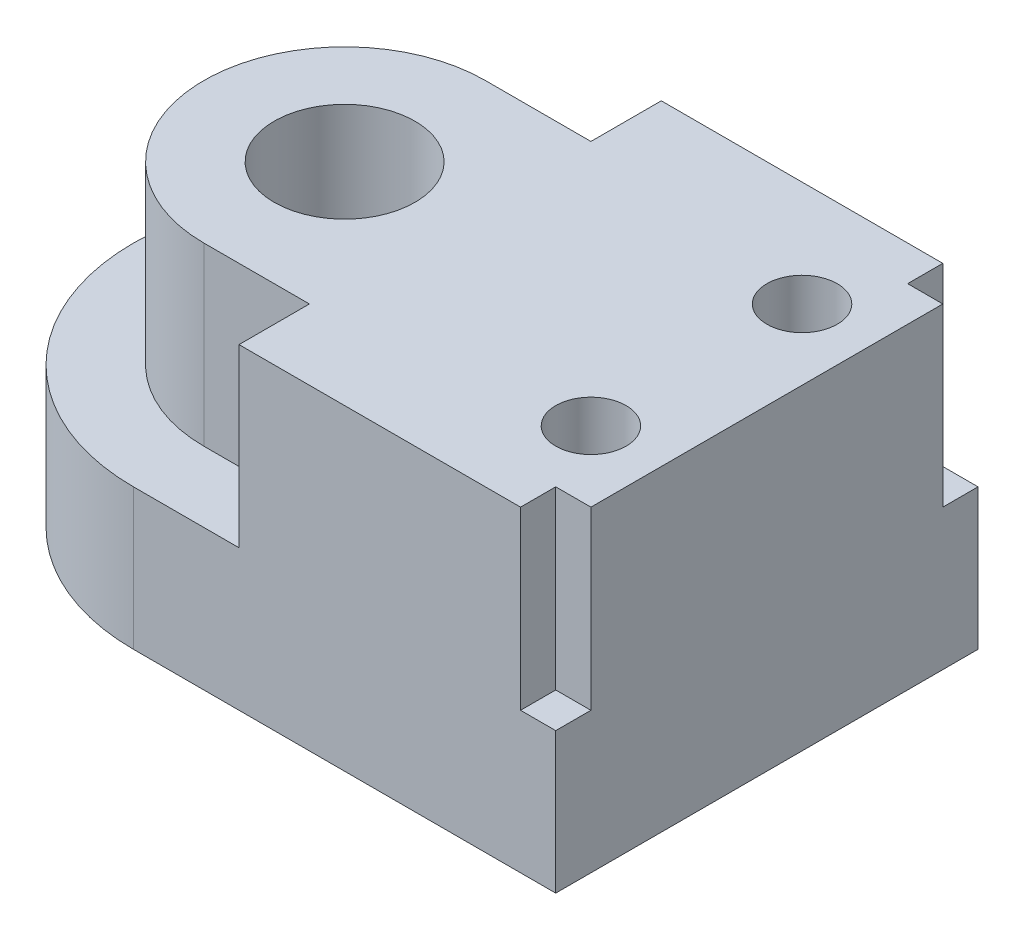
ISO-10303-21;
HEADER;
FILE_DESCRIPTION(('STEP AP214'),'2;1');
FILE_NAME('part.step','',(''),(''),'','','');
FILE_SCHEMA(('AUTOMOTIVE_DESIGN { 1 0 10303 214 1 1 1 1 }'));
ENDSEC;
DATA;
#1=APPLICATION_CONTEXT('core data for automotive mechanical design processes');
#2=APPLICATION_PROTOCOL_DEFINITION('international standard','automotive_design',2000,#1);
#3=PRODUCT_CONTEXT('',#1,'mechanical');
#4=PRODUCT('Part','Part','',(#3));
#5=PRODUCT_RELATED_PRODUCT_CATEGORY('part','',(#4));
#6=PRODUCT_DEFINITION_FORMATION('','',#4);
#7=PRODUCT_DEFINITION_CONTEXT('part definition',#1,'design');
#8=PRODUCT_DEFINITION('design','',#6,#7);
#9=PRODUCT_DEFINITION_SHAPE('','',#8);
#10=(LENGTH_UNIT() NAMED_UNIT(*) SI_UNIT(.MILLI.,.METRE.));
#11=(NAMED_UNIT(*) PLANE_ANGLE_UNIT() SI_UNIT($,.RADIAN.));
#12=(NAMED_UNIT(*) SI_UNIT($,.STERADIAN.) SOLID_ANGLE_UNIT());
#13=UNCERTAINTY_MEASURE_WITH_UNIT(LENGTH_MEASURE(1.E-05),#10,'distance_accuracy_value','');
#14=(GEOMETRIC_REPRESENTATION_CONTEXT(3) GLOBAL_UNCERTAINTY_ASSIGNED_CONTEXT((#13)) GLOBAL_UNIT_ASSIGNED_CONTEXT((#10,
#11,#12)) REPRESENTATION_CONTEXT('',''));
#15=CARTESIAN_POINT('',(0.,0.,0.));
#16=DIRECTION('',(0.,0.,1.));
#17=DIRECTION('',(1.,0.,0.));
#18=AXIS2_PLACEMENT_3D('',#15,#16,#17);
#19=CARTESIAN_POINT('',(-51.6932321042145,20.,-1.39241029236941));
#20=DIRECTION('',(0.,1.,0.));
#21=DIRECTION('',(0.,0.,1.));
#22=AXIS2_PLACEMENT_3D('',#19,#20,#21);
#23=PLANE('',#22);
#24=DIRECTION('',(1.,0.,0.));
#25=VECTOR('',#24,1.);
#26=CARTESIAN_POINT('',(-51.6932321042145,20.,28.6075897076306));
#27=LINE('',#26,#25);
#28=CARTESIAN_POINT('',(-51.6932321042145,20.,28.6075897076306));
#29=VERTEX_POINT('',#28);
#30=CARTESIAN_POINT('',(-36.6932321042145,20.,28.6075897076306));
#31=VERTEX_POINT('',#30);
#32=EDGE_CURVE('E206',#29,#31,#27,.T.);
#33=ORIENTED_EDGE('',*,*,#32,.T.);
#34=DIRECTION('',(0.,0.,1.));
#35=VECTOR('',#34,1.);
#36=CARTESIAN_POINT('',(-36.6932321042145,20.,0.));
#37=LINE('',#36,#35);
#38=CARTESIAN_POINT('',(-36.6932321042145,20.,18.6075897076306));
#39=VERTEX_POINT('',#38);
#40=EDGE_CURVE('E176',#39,#31,#37,.T.);
#41=ORIENTED_EDGE('',*,*,#40,.F.);
#42=DIRECTION('',(1.,0.,0.));
#43=VECTOR('',#42,1.);
#44=CARTESIAN_POINT('',(8.30676789578554,20.,18.6075897076306));
#45=LINE('',#44,#43);
#46=CARTESIAN_POINT('',(-51.6932321042145,20.,18.6075897076306));
#47=VERTEX_POINT('',#46);
#48=EDGE_CURVE('E174',#47,#39,#45,.T.);
#49=ORIENTED_EDGE('',*,*,#48,.F.);
#50=CARTESIAN_POINT('',(-51.6932321042145,20.,-1.39241029236941));
#51=DIRECTION('',(0.,1.,0.));
#52=DIRECTION('',(0.,0.,1.));
#53=AXIS2_PLACEMENT_3D('',#50,#51,#52);
#54=CIRCLE('',#53,20.);
#55=CARTESIAN_POINT('',(-51.6932321042145,20.,-21.3924102923694));
#56=VERTEX_POINT('',#55);
#57=EDGE_CURVE('E197',#56,#47,#54,.T.);
#58=ORIENTED_EDGE('',*,*,#57,.F.);
#59=DIRECTION('',(-1.,0.,0.));
#60=VECTOR('',#59,1.);
#61=CARTESIAN_POINT('',(-51.6932321042145,20.,-21.3924102923694));
#62=LINE('',#61,#60);
#63=CARTESIAN_POINT('',(-36.6932321042145,20.,-21.3924102923694));
#64=VERTEX_POINT('',#63);
#65=EDGE_CURVE('E194',#64,#56,#62,.T.);
#66=ORIENTED_EDGE('',*,*,#65,.F.);
#67=DIRECTION('',(0.,0.,1.));
#68=VECTOR('',#67,1.);
#69=CARTESIAN_POINT('',(-36.6932321042145,20.,0.));
#70=LINE('',#69,#68);
#71=CARTESIAN_POINT('',(-36.6932321042145,20.,-31.3924102923694));
#72=VERTEX_POINT('',#71);
#73=EDGE_CURVE('E246',#72,#64,#70,.T.);
#74=ORIENTED_EDGE('',*,*,#73,.F.);
#75=DIRECTION('',(-1.,0.,0.));
#76=VECTOR('',#75,1.);
#77=CARTESIAN_POINT('',(-51.6932321042145,20.,-31.3924102923694));
#78=LINE('',#77,#76);
#79=CARTESIAN_POINT('',(-51.6932321042145,20.,-31.3924102923694));
#80=VERTEX_POINT('',#79);
#81=EDGE_CURVE('E203',#72,#80,#78,.T.);
#82=ORIENTED_EDGE('',*,*,#81,.T.);
#83=CARTESIAN_POINT('',(-51.6932321042145,20.,-1.39241029236941));
#84=DIRECTION('',(0.,1.,0.));
#85=DIRECTION('',(0.,0.,1.));
#86=AXIS2_PLACEMENT_3D('',#83,#84,#85);
#87=CIRCLE('',#86,30.);
#88=EDGE_CURVE('E204',#80,#29,#87,.T.);
#89=ORIENTED_EDGE('',*,*,#88,.T.);
#90=EDGE_LOOP('',(#33,#41,#49,#58,#66,#74,#82,#89));
#91=FACE_BOUND('',#90,.T.);
#92=ADVANCED_FACE('F41',(#91),#23,.T.);
#93=CARTESIAN_POINT('',(8.30676789578554,20.,18.6075897076306));
#94=DIRECTION('',(0.,0.,1.));
#95=DIRECTION('',(1.,0.,0.));
#96=AXIS2_PLACEMENT_3D('',#93,#94,#95);
#97=PLANE('',#96);
#98=ORIENTED_EDGE('',*,*,#48,.T.);
#99=DIRECTION('',(0.,-1.,0.));
#100=VECTOR('',#99,1.);
#101=CARTESIAN_POINT('',(-36.6932321042145,56.1803398874989,18.6075897076306));
#102=LINE('',#101,#100);
#103=CARTESIAN_POINT('',(-36.6932321042145,45.,18.6075897076306));
#104=VERTEX_POINT('',#103);
#105=EDGE_CURVE('E159',#104,#39,#102,.T.);
#106=ORIENTED_EDGE('',*,*,#105,.F.);
#107=DIRECTION('',(1.,0.,0.));
#108=VECTOR('',#107,1.);
#109=CARTESIAN_POINT('',(0.,45.,18.6075897076306));
#110=LINE('',#109,#108);
#111=CARTESIAN_POINT('',(-51.6932321042145,45.,18.6075897076306));
#112=VERTEX_POINT('',#111);
#113=EDGE_CURVE('E175',#112,#104,#110,.T.);
#114=ORIENTED_EDGE('',*,*,#113,.F.);
#115=DIRECTION('',(0.,1.,0.));
#116=VECTOR('',#115,1.);
#117=CARTESIAN_POINT('',(-51.6932321042145,20.,18.6075897076306));
#118=LINE('',#117,#116);
#119=EDGE_CURVE('E195',#47,#112,#118,.T.);
#120=ORIENTED_EDGE('',*,*,#119,.F.);
#121=EDGE_LOOP('',(#98,#106,#114,#120));
#122=FACE_BOUND('',#121,.T.);
#123=ADVANCED_FACE('F171',(#122),#97,.T.);
#124=CARTESIAN_POINT('',(-51.6932321042145,20.,-21.3924102923694));
#125=DIRECTION('',(0.,0.,-1.));
#126=DIRECTION('',(-1.,0.,0.));
#127=AXIS2_PLACEMENT_3D('',#124,#125,#126);
#128=PLANE('',#127);
#129=DIRECTION('',(-1.,0.,0.));
#130=VECTOR('',#129,1.);
#131=CARTESIAN_POINT('',(0.,45.,-21.3924102923694));
#132=LINE('',#131,#130);
#133=CARTESIAN_POINT('',(-36.6932321042145,45.,-21.3924102923694));
#134=VERTEX_POINT('',#133);
#135=CARTESIAN_POINT('',(-51.6932321042145,45.,-21.3924102923694));
#136=VERTEX_POINT('',#135);
#137=EDGE_CURVE('E182',#134,#136,#132,.T.);
#138=ORIENTED_EDGE('',*,*,#137,.F.);
#139=DIRECTION('',(0.,-1.,0.));
#140=VECTOR('',#139,1.);
#141=CARTESIAN_POINT('',(-36.6932321042145,56.1803398874989,-21.3924102923694));
#142=LINE('',#141,#140);
#143=EDGE_CURVE('E254',#134,#64,#142,.T.);
#144=ORIENTED_EDGE('',*,*,#143,.T.);
#145=ORIENTED_EDGE('',*,*,#65,.T.);
#146=DIRECTION('',(0.,1.,0.));
#147=VECTOR('',#146,1.);
#148=CARTESIAN_POINT('',(-51.6932321042145,20.,-21.3924102923694));
#149=LINE('',#148,#147);
#150=EDGE_CURVE('E191',#56,#136,#149,.T.);
#151=ORIENTED_EDGE('',*,*,#150,.T.);
#152=EDGE_LOOP('',(#138,#144,#145,#151));
#153=FACE_BOUND('',#152,.T.);
#154=ADVANCED_FACE('F325',(#153),#128,.T.);
#155=CARTESIAN_POINT('',(8.30676789578554,20.,-1.39241029236941));
#156=DIRECTION('',(-1.,0.,0.));
#157=DIRECTION('',(0.,0.,1.));
#158=AXIS2_PLACEMENT_3D('',#155,#156,#157);
#159=PLANE('',#158);
#160=DIRECTION('',(0.,0.,-1.));
#161=VECTOR('',#160,1.);
#162=CARTESIAN_POINT('',(8.30676789578554,45.,0.));
#163=LINE('',#162,#161);
#164=CARTESIAN_POINT('',(8.30676789578554,45.,23.6075897076306));
#165=VERTEX_POINT('',#164);
#166=CARTESIAN_POINT('',(8.30676789578554,45.,-26.3924102923694));
#167=VERTEX_POINT('',#166);
#168=EDGE_CURVE('E185',#165,#167,#163,.T.);
#169=ORIENTED_EDGE('',*,*,#168,.F.);
#170=DIRECTION('',(0.,1.,0.));
#171=VECTOR('',#170,1.);
#172=CARTESIAN_POINT('',(8.30676789578554,20.,23.6075897076306));
#173=LINE('',#172,#171);
#174=CARTESIAN_POINT('',(8.30676789578554,20.,23.6075897076306));
#175=VERTEX_POINT('',#174);
#176=EDGE_CURVE('E60',#175,#165,#173,.T.);
#177=ORIENTED_EDGE('',*,*,#176,.F.);
#178=DIRECTION('',(0.,0.,-1.));
#179=VECTOR('',#178,1.);
#180=CARTESIAN_POINT('',(8.30676789578554,20.,28.6075897076306));
#181=LINE('',#180,#179);
#182=CARTESIAN_POINT('',(8.30676789578554,20.,28.6075897076306));
#183=VERTEX_POINT('',#182);
#184=EDGE_CURVE('E269',#183,#175,#181,.T.);
#185=ORIENTED_EDGE('',*,*,#184,.F.);
#186=DIRECTION('',(0.,-1.,0.));
#187=VECTOR('',#186,1.);
#188=CARTESIAN_POINT('',(8.30676789578554,20.,28.6075897076306));
#189=LINE('',#188,#187);
#190=CARTESIAN_POINT('',(8.30676789578554,0.,28.6075897076306));
#191=VERTEX_POINT('',#190);
#192=EDGE_CURVE('E213',#183,#191,#189,.T.);
#193=ORIENTED_EDGE('',*,*,#192,.T.);
#194=DIRECTION('',(0.,0.,-1.));
#195=VECTOR('',#194,1.);
#196=CARTESIAN_POINT('',(8.30676789578554,0.,-1.39241029236941));
#197=LINE('',#196,#195);
#198=CARTESIAN_POINT('',(8.30676789578554,0.,-31.3924102923694));
#199=VERTEX_POINT('',#198);
#200=EDGE_CURVE('E205',#191,#199,#197,.T.);
#201=ORIENTED_EDGE('',*,*,#200,.T.);
#202=DIRECTION('',(0.,-1.,0.));
#203=VECTOR('',#202,1.);
#204=CARTESIAN_POINT('',(8.30676789578554,20.,-31.3924102923694));
#205=LINE('',#204,#203);
#206=CARTESIAN_POINT('',(8.30676789578554,20.,-31.3924102923694));
#207=VERTEX_POINT('',#206);
#208=EDGE_CURVE('E11',#207,#199,#205,.T.);
#209=ORIENTED_EDGE('',*,*,#208,.F.);
#210=DIRECTION('',(0.,0.,-1.));
#211=VECTOR('',#210,1.);
#212=CARTESIAN_POINT('',(8.30676789578554,20.,-31.3924102923694));
#213=LINE('',#212,#211);
#214=CARTESIAN_POINT('',(8.30676789578554,20.,-26.3924102923694));
#215=VERTEX_POINT('',#214);
#216=EDGE_CURVE('E293',#215,#207,#213,.T.);
#217=ORIENTED_EDGE('',*,*,#216,.F.);
#218=DIRECTION('',(0.,1.,0.));
#219=VECTOR('',#218,1.);
#220=CARTESIAN_POINT('',(8.30676789578554,20.,-26.3924102923694));
#221=LINE('',#220,#219);
#222=EDGE_CURVE('E306',#215,#167,#221,.T.);
#223=ORIENTED_EDGE('',*,*,#222,.T.);
#224=EDGE_LOOP('',(#169,#177,#185,#193,#201,#209,#217,#223));
#225=FACE_BOUND('',#224,.T.);
#226=ADVANCED_FACE('F43',(#225),#159,.F.);
#227=CARTESIAN_POINT('',(-51.6932321042145,20.,-31.3924102923694));
#228=DIRECTION('',(0.,0.,1.));
#229=DIRECTION('',(1.,0.,0.));
#230=AXIS2_PLACEMENT_3D('',#227,#228,#229);
#231=PLANE('',#230);
#232=ORIENTED_EDGE('',*,*,#81,.F.);
#233=DIRECTION('',(0.,-1.,0.));
#234=VECTOR('',#233,1.);
#235=CARTESIAN_POINT('',(-36.6932321042145,56.1803398874989,-31.3924102923694));
#236=LINE('',#235,#234);
#237=CARTESIAN_POINT('',(-36.6932321042145,45.,-31.3924102923694));
#238=VERTEX_POINT('',#237);
#239=EDGE_CURVE('E168',#238,#72,#236,.T.);
#240=ORIENTED_EDGE('',*,*,#239,.F.);
#241=DIRECTION('',(-1.,0.,0.));
#242=VECTOR('',#241,1.);
#243=CARTESIAN_POINT('',(8.30676789578554,45.,-31.3924102923694));
#244=LINE('',#243,#242);
#245=CARTESIAN_POINT('',(3.30676789578554,45.,-31.3924102923694));
#246=VERTEX_POINT('',#245);
#247=EDGE_CURVE('E187',#246,#238,#244,.T.);
#248=ORIENTED_EDGE('',*,*,#247,.F.);
#249=DIRECTION('',(0.,1.,0.));
#250=VECTOR('',#249,1.);
#251=CARTESIAN_POINT('',(3.30676789578554,20.,-31.3924102923694));
#252=LINE('',#251,#250);
#253=CARTESIAN_POINT('',(3.30676789578554,20.,-31.3924102923694));
#254=VERTEX_POINT('',#253);
#255=EDGE_CURVE('E61',#254,#246,#252,.T.);
#256=ORIENTED_EDGE('',*,*,#255,.F.);
#257=DIRECTION('',(-1.,0.,0.));
#258=VECTOR('',#257,1.);
#259=CARTESIAN_POINT('',(8.30676789578554,20.,-31.3924102923694));
#260=LINE('',#259,#258);
#261=EDGE_CURVE('E291',#207,#254,#260,.T.);
#262=ORIENTED_EDGE('',*,*,#261,.F.);
#263=ORIENTED_EDGE('',*,*,#208,.T.);
#264=DIRECTION('',(-1.,0.,0.));
#265=VECTOR('',#264,1.);
#266=CARTESIAN_POINT('',(-51.6932321042145,0.,-31.3924102923694));
#267=LINE('',#266,#265);
#268=CARTESIAN_POINT('',(-51.6932321042145,0.,-31.3924102923694));
#269=VERTEX_POINT('',#268);
#270=EDGE_CURVE('E215',#199,#269,#267,.T.);
#271=ORIENTED_EDGE('',*,*,#270,.T.);
#272=DIRECTION('',(0.,-1.,0.));
#273=VECTOR('',#272,1.);
#274=CARTESIAN_POINT('',(-51.6932321042145,20.,-31.3924102923694));
#275=LINE('',#274,#273);
#276=EDGE_CURVE('E49',#80,#269,#275,.T.);
#277=ORIENTED_EDGE('',*,*,#276,.F.);
#278=EDGE_LOOP('',(#232,#240,#248,#256,#262,#263,#271,#277));
#279=FACE_BOUND('',#278,.T.);
#280=ADVANCED_FACE('F247',(#279),#231,.F.);
#281=CARTESIAN_POINT('',(-51.6932321042145,20.,-1.39241029236941));
#282=DIRECTION('',(0.,-1.,0.));
#283=DIRECTION('',(0.,0.,-1.));
#284=AXIS2_PLACEMENT_3D('',#281,#282,#283);
#285=CYLINDRICAL_SURFACE('',#284,30.);
#286=CARTESIAN_POINT('',(-51.6932321042145,0.,-1.39241029236941));
#287=DIRECTION('',(0.,1.,0.));
#288=DIRECTION('',(0.,0.,1.));
#289=AXIS2_PLACEMENT_3D('',#286,#287,#288);
#290=CIRCLE('',#289,30.);
#291=CARTESIAN_POINT('',(-51.6932321042145,0.,28.6075897076306));
#292=VERTEX_POINT('',#291);
#293=EDGE_CURVE('E216',#269,#292,#290,.T.);
#294=ORIENTED_EDGE('',*,*,#293,.T.);
#295=DIRECTION('',(0.,-1.,0.));
#296=VECTOR('',#295,1.);
#297=CARTESIAN_POINT('',(-51.6932321042145,20.,28.6075897076306));
#298=LINE('',#297,#296);
#299=EDGE_CURVE('E221',#29,#292,#298,.T.);
#300=ORIENTED_EDGE('',*,*,#299,.F.);
#301=ORIENTED_EDGE('',*,*,#88,.F.);
#302=ORIENTED_EDGE('',*,*,#276,.T.);
#303=EDGE_LOOP('',(#294,#300,#301,#302));
#304=FACE_BOUND('',#303,.T.);
#305=ADVANCED_FACE('F230',(#304),#285,.T.);
#306=CARTESIAN_POINT('',(-51.6932321042145,20.,28.6075897076306));
#307=DIRECTION('',(0.,0.,-1.));
#308=DIRECTION('',(-1.,0.,0.));
#309=AXIS2_PLACEMENT_3D('',#306,#307,#308);
#310=PLANE('',#309);
#311=DIRECTION('',(1.,0.,0.));
#312=VECTOR('',#311,1.);
#313=CARTESIAN_POINT('',(8.30676789578554,20.,28.6075897076306));
#314=LINE('',#313,#312);
#315=CARTESIAN_POINT('',(3.30676789578554,20.,28.6075897076306));
#316=VERTEX_POINT('',#315);
#317=EDGE_CURVE('E276',#316,#183,#314,.T.);
#318=ORIENTED_EDGE('',*,*,#317,.F.);
#319=DIRECTION('',(0.,1.,0.));
#320=VECTOR('',#319,1.);
#321=CARTESIAN_POINT('',(3.30676789578554,20.,28.6075897076306));
#322=LINE('',#321,#320);
#323=CARTESIAN_POINT('',(3.30676789578554,45.,28.6075897076306));
#324=VERTEX_POINT('',#323);
#325=EDGE_CURVE('E283',#316,#324,#322,.T.);
#326=ORIENTED_EDGE('',*,*,#325,.T.);
#327=DIRECTION('',(1.,0.,0.));
#328=VECTOR('',#327,1.);
#329=CARTESIAN_POINT('',(8.30676789578554,45.,28.6075897076306));
#330=LINE('',#329,#328);
#331=CARTESIAN_POINT('',(-36.6932321042145,45.,28.6075897076306));
#332=VERTEX_POINT('',#331);
#333=EDGE_CURVE('E319',#332,#324,#330,.T.);
#334=ORIENTED_EDGE('',*,*,#333,.F.);
#335=DIRECTION('',(0.,-1.,0.));
#336=VECTOR('',#335,1.);
#337=CARTESIAN_POINT('',(-36.6932321042145,56.1803398874989,28.6075897076306));
#338=LINE('',#337,#336);
#339=EDGE_CURVE('E162',#332,#31,#338,.T.);
#340=ORIENTED_EDGE('',*,*,#339,.T.);
#341=ORIENTED_EDGE('',*,*,#32,.F.);
#342=ORIENTED_EDGE('',*,*,#299,.T.);
#343=DIRECTION('',(1.,0.,0.));
#344=VECTOR('',#343,1.);
#345=CARTESIAN_POINT('',(-51.6932321042145,0.,28.6075897076306));
#346=LINE('',#345,#344);
#347=EDGE_CURVE('E207',#292,#191,#346,.T.);
#348=ORIENTED_EDGE('',*,*,#347,.T.);
#349=ORIENTED_EDGE('',*,*,#192,.F.);
#350=EDGE_LOOP('',(#318,#326,#334,#340,#341,#342,#348,#349));
#351=FACE_BOUND('',#350,.T.);
#352=ADVANCED_FACE('F241',(#351),#310,.F.);
#353=CARTESIAN_POINT('',(-51.6932321042145,0.,-1.39241029236941));
#354=DIRECTION('',(0.,1.,0.));
#355=DIRECTION('',(0.,0.,1.));
#356=AXIS2_PLACEMENT_3D('',#353,#354,#355);
#357=PLANE('',#356);
#358=CARTESIAN_POINT('',(-1.69323210421446,0.,-16.3924102923694));
#359=DIRECTION('',(0.,1.,0.));
#360=DIRECTION('',(0.,0.,1.));
#361=AXIS2_PLACEMENT_3D('',#358,#359,#360);
#362=CIRCLE('',#361,5.);
#363=CARTESIAN_POINT('',(-1.69323210421446,0.,-11.3924102923694));
#364=VERTEX_POINT('',#363);
#365=EDGE_CURVE('E262',#364,#364,#362,.T.);
#366=ORIENTED_EDGE('',*,*,#365,.T.);
#367=EDGE_LOOP('',(#366));
#368=FACE_BOUND('',#367,.T.);
#369=CARTESIAN_POINT('',(-1.69323210421446,0.,13.6075897076306));
#370=DIRECTION('',(0.,1.,0.));
#371=DIRECTION('',(0.,0.,1.));
#372=AXIS2_PLACEMENT_3D('',#369,#370,#371);
#373=CIRCLE('',#372,5.);
#374=CARTESIAN_POINT('',(-1.69323210421446,0.,18.6075897076306));
#375=VERTEX_POINT('',#374);
#376=EDGE_CURVE('E266',#375,#375,#373,.F.);
#377=ORIENTED_EDGE('',*,*,#376,.F.);
#378=EDGE_LOOP('',(#377));
#379=FACE_BOUND('',#378,.T.);
#380=CARTESIAN_POINT('',(-51.6932321042145,0.,-1.39241029236941));
#381=DIRECTION('',(0.,1.,0.));
#382=DIRECTION('',(0.,0.,1.));
#383=AXIS2_PLACEMENT_3D('',#380,#381,#382);
#384=CIRCLE('',#383,10.);
#385=CARTESIAN_POINT('',(-51.6932321042145,0.,8.60758970763059));
#386=VERTEX_POINT('',#385);
#387=EDGE_CURVE('E314',#386,#386,#384,.T.);
#388=ORIENTED_EDGE('',*,*,#387,.T.);
#389=EDGE_LOOP('',(#388));
#390=FACE_BOUND('',#389,.T.);
#391=ORIENTED_EDGE('',*,*,#200,.F.);
#392=ORIENTED_EDGE('',*,*,#347,.F.);
#393=ORIENTED_EDGE('',*,*,#293,.F.);
#394=ORIENTED_EDGE('',*,*,#270,.F.);
#395=EDGE_LOOP('',(#391,#392,#393,#394));
#396=FACE_BOUND('',#395,.T.);
#397=ADVANCED_FACE('F240',(#368,#379,#390,#396),#357,.F.);
#398=CARTESIAN_POINT('',(-51.6932321042145,25.,-1.39241029236941));
#399=DIRECTION('',(0.,-1.,0.));
#400=DIRECTION('',(0.,0.,-1.));
#401=AXIS2_PLACEMENT_3D('',#398,#399,#400);
#402=CYLINDRICAL_SURFACE('',#401,20.);
#403=CARTESIAN_POINT('',(-51.6932321042145,45.,-1.39241029236941));
#404=DIRECTION('',(0.,1.,0.));
#405=DIRECTION('',(0.,0.,1.));
#406=AXIS2_PLACEMENT_3D('',#403,#404,#405);
#407=CIRCLE('',#406,20.);
#408=EDGE_CURVE('E181',#136,#112,#407,.T.);
#409=ORIENTED_EDGE('',*,*,#408,.F.);
#410=ORIENTED_EDGE('',*,*,#150,.F.);
#411=ORIENTED_EDGE('',*,*,#57,.T.);
#412=ORIENTED_EDGE('',*,*,#119,.T.);
#413=EDGE_LOOP('',(#409,#410,#411,#412));
#414=FACE_BOUND('',#413,.T.);
#415=ADVANCED_FACE('F327',(#414),#402,.T.);
#416=CARTESIAN_POINT('',(-51.6932321042145,45.,-1.39241029236941));
#417=DIRECTION('',(0.,1.,0.));
#418=DIRECTION('',(0.,0.,1.));
#419=AXIS2_PLACEMENT_3D('',#416,#417,#418);
#420=PLANE('',#419);
#421=ORIENTED_EDGE('',*,*,#113,.T.);
#422=DIRECTION('',(0.,0.,1.));
#423=VECTOR('',#422,1.);
#424=CARTESIAN_POINT('',(-36.6932321042145,45.,0.));
#425=LINE('',#424,#423);
#426=EDGE_CURVE('E156',#104,#332,#425,.T.);
#427=ORIENTED_EDGE('',*,*,#426,.T.);
#428=ORIENTED_EDGE('',*,*,#333,.T.);
#429=DIRECTION('',(0.,0.,1.));
#430=VECTOR('',#429,1.);
#431=CARTESIAN_POINT('',(3.30676789578554,45.,28.6075897076306));
#432=LINE('',#431,#430);
#433=CARTESIAN_POINT('',(3.30676789578554,45.,23.6075897076306));
#434=VERTEX_POINT('',#433);
#435=EDGE_CURVE('E274',#434,#324,#432,.T.);
#436=ORIENTED_EDGE('',*,*,#435,.F.);
#437=DIRECTION('',(-1.,0.,0.));
#438=VECTOR('',#437,1.);
#439=CARTESIAN_POINT('',(8.30676789578554,45.,23.6075897076306));
#440=LINE('',#439,#438);
#441=EDGE_CURVE('E267',#165,#434,#440,.T.);
#442=ORIENTED_EDGE('',*,*,#441,.F.);
#443=ORIENTED_EDGE('',*,*,#168,.T.);
#444=DIRECTION('',(1.,0.,0.));
#445=VECTOR('',#444,1.);
#446=CARTESIAN_POINT('',(8.30676789578554,45.,-26.3924102923694));
#447=LINE('',#446,#445);
#448=CARTESIAN_POINT('',(3.30676789578554,45.,-26.3924102923694));
#449=VERTEX_POINT('',#448);
#450=EDGE_CURVE('E295',#449,#167,#447,.T.);
#451=ORIENTED_EDGE('',*,*,#450,.F.);
#452=DIRECTION('',(0.,0.,1.));
#453=VECTOR('',#452,1.);
#454=CARTESIAN_POINT('',(3.30676789578554,45.,-31.3924102923694));
#455=LINE('',#454,#453);
#456=EDGE_CURVE('E290',#246,#449,#455,.T.);
#457=ORIENTED_EDGE('',*,*,#456,.F.);
#458=ORIENTED_EDGE('',*,*,#247,.T.);
#459=DIRECTION('',(0.,0.,1.));
#460=VECTOR('',#459,1.);
#461=CARTESIAN_POINT('',(-36.6932321042145,45.,0.));
#462=LINE('',#461,#460);
#463=EDGE_CURVE('E259',#238,#134,#462,.T.);
#464=ORIENTED_EDGE('',*,*,#463,.T.);
#465=ORIENTED_EDGE('',*,*,#137,.T.);
#466=ORIENTED_EDGE('',*,*,#408,.T.);
#467=EDGE_LOOP('',(#421,#427,#428,#436,#442,#443,#451,#457,#458,#464,#465,#466));
#468=FACE_BOUND('',#467,.T.);
#469=CARTESIAN_POINT('',(-1.69323210421446,45.,-16.3924102923694));
#470=DIRECTION('',(0.,1.,0.));
#471=DIRECTION('',(0.,0.,1.));
#472=AXIS2_PLACEMENT_3D('',#469,#470,#471);
#473=CIRCLE('',#472,5.);
#474=CARTESIAN_POINT('',(-1.69323210421446,45.,-11.3924102923694));
#475=VERTEX_POINT('',#474);
#476=EDGE_CURVE('E256',#475,#475,#473,.T.);
#477=ORIENTED_EDGE('',*,*,#476,.F.);
#478=EDGE_LOOP('',(#477));
#479=FACE_BOUND('',#478,.T.);
#480=CARTESIAN_POINT('',(-1.69323210421446,45.,13.6075897076306));
#481=DIRECTION('',(0.,1.,0.));
#482=DIRECTION('',(0.,0.,1.));
#483=AXIS2_PLACEMENT_3D('',#480,#481,#482);
#484=CIRCLE('',#483,5.);
#485=CARTESIAN_POINT('',(-1.69323210421446,45.,18.6075897076306));
#486=VERTEX_POINT('',#485);
#487=EDGE_CURVE('E44',#486,#486,#484,.F.);
#488=ORIENTED_EDGE('',*,*,#487,.T.);
#489=EDGE_LOOP('',(#488));
#490=FACE_BOUND('',#489,.T.);
#491=CARTESIAN_POINT('',(-51.6932321042145,45.,-1.39241029236941));
#492=DIRECTION('',(0.,1.,0.));
#493=DIRECTION('',(0.,0.,1.));
#494=AXIS2_PLACEMENT_3D('',#491,#492,#493);
#495=CIRCLE('',#494,10.);
#496=CARTESIAN_POINT('',(-51.6932321042145,45.,8.60758970763059));
#497=VERTEX_POINT('',#496);
#498=EDGE_CURVE('E307',#497,#497,#495,.T.);
#499=ORIENTED_EDGE('',*,*,#498,.F.);
#500=EDGE_LOOP('',(#499));
#501=FACE_BOUND('',#500,.T.);
#502=ADVANCED_FACE('F178',(#468,#479,#490,#501),#420,.T.);
#503=CARTESIAN_POINT('',(-51.6932321042145,-31.,-1.39241029236941));
#504=DIRECTION('',(0.,1.,0.));
#505=DIRECTION('',(0.,0.,1.));
#506=AXIS2_PLACEMENT_3D('',#503,#504,#505);
#507=CYLINDRICAL_SURFACE('',#506,10.);
#508=ORIENTED_EDGE('',*,*,#498,.T.);
#509=EDGE_LOOP('',(#508));
#510=FACE_BOUND('',#509,.T.);
#511=ORIENTED_EDGE('',*,*,#387,.F.);
#512=EDGE_LOOP('',(#511));
#513=FACE_BOUND('',#512,.T.);
#514=ADVANCED_FACE('F337',(#510,#513),#507,.F.);
#515=CARTESIAN_POINT('',(8.30676789578554,20.,-26.3924102923694));
#516=DIRECTION('',(0.,0.,1.));
#517=DIRECTION('',(1.,0.,0.));
#518=AXIS2_PLACEMENT_3D('',#515,#516,#517);
#519=PLANE('',#518);
#520=ORIENTED_EDGE('',*,*,#450,.T.);
#521=ORIENTED_EDGE('',*,*,#222,.F.);
#522=DIRECTION('',(1.,0.,0.));
#523=VECTOR('',#522,1.);
#524=CARTESIAN_POINT('',(8.30676789578554,20.,-26.3924102923694));
#525=LINE('',#524,#523);
#526=CARTESIAN_POINT('',(3.30676789578554,20.,-26.3924102923694));
#527=VERTEX_POINT('',#526);
#528=EDGE_CURVE('E297',#527,#215,#525,.T.);
#529=ORIENTED_EDGE('',*,*,#528,.F.);
#530=DIRECTION('',(0.,1.,0.));
#531=VECTOR('',#530,1.);
#532=CARTESIAN_POINT('',(3.30676789578554,20.,-26.3924102923694));
#533=LINE('',#532,#531);
#534=EDGE_CURVE('E309',#527,#449,#533,.T.);
#535=ORIENTED_EDGE('',*,*,#534,.T.);
#536=EDGE_LOOP('',(#520,#521,#529,#535));
#537=FACE_BOUND('',#536,.T.);
#538=ADVANCED_FACE('F370',(#537),#519,.F.);
#539=CARTESIAN_POINT('',(3.30676789578554,20.,-31.3924102923694));
#540=DIRECTION('',(-1.,0.,0.));
#541=DIRECTION('',(0.,0.,1.));
#542=AXIS2_PLACEMENT_3D('',#539,#540,#541);
#543=PLANE('',#542);
#544=ORIENTED_EDGE('',*,*,#456,.T.);
#545=ORIENTED_EDGE('',*,*,#534,.F.);
#546=DIRECTION('',(0.,0.,1.));
#547=VECTOR('',#546,1.);
#548=CARTESIAN_POINT('',(3.30676789578554,20.,-31.3924102923694));
#549=LINE('',#548,#547);
#550=EDGE_CURVE('E300',#254,#527,#549,.T.);
#551=ORIENTED_EDGE('',*,*,#550,.F.);
#552=ORIENTED_EDGE('',*,*,#255,.T.);
#553=EDGE_LOOP('',(#544,#545,#551,#552));
#554=FACE_BOUND('',#553,.T.);
#555=ADVANCED_FACE('F367',(#554),#543,.F.);
#556=CARTESIAN_POINT('',(0.,20.,0.));
#557=DIRECTION('',(0.,-1.,0.));
#558=DIRECTION('',(0.,0.,-1.));
#559=AXIS2_PLACEMENT_3D('',#556,#557,#558);
#560=PLANE('',#559);
#561=ORIENTED_EDGE('',*,*,#216,.T.);
#562=ORIENTED_EDGE('',*,*,#261,.T.);
#563=ORIENTED_EDGE('',*,*,#550,.T.);
#564=ORIENTED_EDGE('',*,*,#528,.T.);
#565=EDGE_LOOP('',(#561,#562,#563,#564));
#566=FACE_BOUND('',#565,.T.);
#567=ADVANCED_FACE('F371',(#566),#560,.F.);
#568=CARTESIAN_POINT('',(3.30676789578554,20.,28.6075897076306));
#569=DIRECTION('',(-1.,0.,0.));
#570=DIRECTION('',(0.,0.,1.));
#571=AXIS2_PLACEMENT_3D('',#568,#569,#570);
#572=PLANE('',#571);
#573=ORIENTED_EDGE('',*,*,#435,.T.);
#574=ORIENTED_EDGE('',*,*,#325,.F.);
#575=DIRECTION('',(0.,0.,1.));
#576=VECTOR('',#575,1.);
#577=CARTESIAN_POINT('',(3.30676789578554,20.,28.6075897076306));
#578=LINE('',#577,#576);
#579=CARTESIAN_POINT('',(3.30676789578554,20.,23.6075897076306));
#580=VERTEX_POINT('',#579);
#581=EDGE_CURVE('E279',#580,#316,#578,.T.);
#582=ORIENTED_EDGE('',*,*,#581,.F.);
#583=DIRECTION('',(0.,1.,0.));
#584=VECTOR('',#583,1.);
#585=CARTESIAN_POINT('',(3.30676789578554,20.,23.6075897076306));
#586=LINE('',#585,#584);
#587=EDGE_CURVE('E288',#580,#434,#586,.T.);
#588=ORIENTED_EDGE('',*,*,#587,.T.);
#589=EDGE_LOOP('',(#573,#574,#582,#588));
#590=FACE_BOUND('',#589,.T.);
#591=ADVANCED_FACE('F376',(#590),#572,.F.);
#592=CARTESIAN_POINT('',(8.30676789578554,20.,23.6075897076306));
#593=DIRECTION('',(0.,0.,-1.));
#594=DIRECTION('',(-1.,0.,0.));
#595=AXIS2_PLACEMENT_3D('',#592,#593,#594);
#596=PLANE('',#595);
#597=ORIENTED_EDGE('',*,*,#441,.T.);
#598=ORIENTED_EDGE('',*,*,#587,.F.);
#599=DIRECTION('',(-1.,0.,0.));
#600=VECTOR('',#599,1.);
#601=CARTESIAN_POINT('',(8.30676789578554,20.,23.6075897076306));
#602=LINE('',#601,#600);
#603=EDGE_CURVE('E271',#175,#580,#602,.T.);
#604=ORIENTED_EDGE('',*,*,#603,.F.);
#605=ORIENTED_EDGE('',*,*,#176,.T.);
#606=EDGE_LOOP('',(#597,#598,#604,#605));
#607=FACE_BOUND('',#606,.T.);
#608=ADVANCED_FACE('F413',(#607),#596,.F.);
#609=CARTESIAN_POINT('',(0.,20.,0.));
#610=DIRECTION('',(0.,1.,0.));
#611=DIRECTION('',(0.,0.,1.));
#612=AXIS2_PLACEMENT_3D('',#609,#610,#611);
#613=PLANE('',#612);
#614=ORIENTED_EDGE('',*,*,#184,.T.);
#615=ORIENTED_EDGE('',*,*,#603,.T.);
#616=ORIENTED_EDGE('',*,*,#581,.T.);
#617=ORIENTED_EDGE('',*,*,#317,.T.);
#618=EDGE_LOOP('',(#614,#615,#616,#617));
#619=FACE_BOUND('',#618,.T.);
#620=ADVANCED_FACE('F425',(#619),#613,.T.);
#621=CARTESIAN_POINT('',(-1.69323210421446,61.,13.6075897076306));
#622=DIRECTION('',(0.,-1.,0.));
#623=DIRECTION('',(0.,0.,-1.));
#624=AXIS2_PLACEMENT_3D('',#621,#622,#623);
#625=CYLINDRICAL_SURFACE('',#624,5.);
#626=ORIENTED_EDGE('',*,*,#487,.F.);
#627=EDGE_LOOP('',(#626));
#628=FACE_BOUND('',#627,.T.);
#629=ORIENTED_EDGE('',*,*,#376,.T.);
#630=EDGE_LOOP('',(#629));
#631=FACE_BOUND('',#630,.T.);
#632=ADVANCED_FACE('F433',(#628,#631),#625,.F.);
#633=CARTESIAN_POINT('',(-1.69323210421446,-77.,-16.3924102923694));
#634=DIRECTION('',(0.,1.,0.));
#635=DIRECTION('',(0.,0.,1.));
#636=AXIS2_PLACEMENT_3D('',#633,#634,#635);
#637=CYLINDRICAL_SURFACE('',#636,5.);
#638=CARTESIAN_POINT('',(-1.69323210421446,45.,-11.3924102923694));
#639=CARTESIAN_POINT('',(-1.69323210421446,44.53125,-11.3924102923694));
#640=CARTESIAN_POINT('',(-1.69323210421446,44.0625,-11.3924102923694));
#641=CARTESIAN_POINT('',(-1.69323210421446,43.125,-11.3924102923694));
#642=CARTESIAN_POINT('',(-1.69323210421446,42.65625,-11.3924102923694));
#643=CARTESIAN_POINT('',(-1.69323210421446,41.71875,-11.3924102923694));
#644=CARTESIAN_POINT('',(-1.69323210421446,41.25,-11.3924102923694));
#645=CARTESIAN_POINT('',(-1.69323210421446,40.3125,-11.3924102923694));
#646=CARTESIAN_POINT('',(-1.69323210421446,39.84375,-11.3924102923694));
#647=CARTESIAN_POINT('',(-1.69323210421446,38.90625,-11.3924102923694));
#648=CARTESIAN_POINT('',(-1.69323210421446,38.4375,-11.3924102923694));
#649=CARTESIAN_POINT('',(-1.69323210421446,37.5,-11.3924102923694));
#650=CARTESIAN_POINT('',(-1.69323210421446,37.03125,-11.3924102923694));
#651=CARTESIAN_POINT('',(-1.69323210421446,36.09375,-11.3924102923694));
#652=CARTESIAN_POINT('',(-1.69323210421446,35.625,-11.3924102923694));
#653=CARTESIAN_POINT('',(-1.69323210421446,34.6875,-11.3924102923694));
#654=CARTESIAN_POINT('',(-1.69323210421446,34.21875,-11.3924102923694));
#655=CARTESIAN_POINT('',(-1.69323210421446,33.28125,-11.3924102923694));
#656=CARTESIAN_POINT('',(-1.69323210421446,32.8125,-11.3924102923694));
#657=CARTESIAN_POINT('',(-1.69323210421446,31.875,-11.3924102923694));
#658=CARTESIAN_POINT('',(-1.69323210421446,31.40625,-11.3924102923694));
#659=CARTESIAN_POINT('',(-1.69323210421446,30.46875,-11.3924102923694));
#660=CARTESIAN_POINT('',(-1.69323210421446,30.,-11.3924102923694));
#661=CARTESIAN_POINT('',(-1.69323210421446,29.0625,-11.3924102923694));
#662=CARTESIAN_POINT('',(-1.69323210421446,28.59375,-11.3924102923694));
#663=CARTESIAN_POINT('',(-1.69323210421446,27.65625,-11.3924102923694));
#664=CARTESIAN_POINT('',(-1.69323210421446,27.1875,-11.3924102923694));
#665=CARTESIAN_POINT('',(-1.69323210421446,26.25,-11.3924102923694));
#666=CARTESIAN_POINT('',(-1.69323210421446,25.78125,-11.3924102923694));
#667=CARTESIAN_POINT('',(-1.69323210421446,24.84375,-11.3924102923694));
#668=CARTESIAN_POINT('',(-1.69323210421446,24.375,-11.3924102923694));
#669=CARTESIAN_POINT('',(-1.69323210421446,23.4375,-11.3924102923694));
#670=CARTESIAN_POINT('',(-1.69323210421446,22.96875,-11.3924102923694));
#671=CARTESIAN_POINT('',(-1.69323210421446,22.03125,-11.3924102923694));
#672=CARTESIAN_POINT('',(-1.69323210421446,21.5625,-11.3924102923694));
#673=CARTESIAN_POINT('',(-1.69323210421446,20.625,-11.3924102923694));
#674=CARTESIAN_POINT('',(-1.69323210421446,20.15625,-11.3924102923694));
#675=CARTESIAN_POINT('',(-1.69323210421446,19.21875,-11.3924102923694));
#676=CARTESIAN_POINT('',(-1.69323210421446,18.75,-11.3924102923694));
#677=CARTESIAN_POINT('',(-1.69323210421446,17.8125,-11.3924102923694));
#678=CARTESIAN_POINT('',(-1.69323210421446,17.34375,-11.3924102923694));
#679=CARTESIAN_POINT('',(-1.69323210421446,16.40625,-11.3924102923694));
#680=CARTESIAN_POINT('',(-1.69323210421446,15.9375,-11.3924102923694));
#681=CARTESIAN_POINT('',(-1.69323210421446,15.,-11.3924102923694));
#682=CARTESIAN_POINT('',(-1.69323210421446,14.53125,-11.3924102923694));
#683=CARTESIAN_POINT('',(-1.69323210421446,13.59375,-11.3924102923694));
#684=CARTESIAN_POINT('',(-1.69323210421446,13.125,-11.3924102923694));
#685=CARTESIAN_POINT('',(-1.69323210421446,12.1875,-11.3924102923694));
#686=CARTESIAN_POINT('',(-1.69323210421446,11.71875,-11.3924102923694));
#687=CARTESIAN_POINT('',(-1.69323210421446,10.78125,-11.3924102923694));
#688=CARTESIAN_POINT('',(-1.69323210421446,10.3125,-11.3924102923694));
#689=CARTESIAN_POINT('',(-1.69323210421446,9.375,-11.3924102923694));
#690=CARTESIAN_POINT('',(-1.69323210421446,8.90625,-11.3924102923694));
#691=CARTESIAN_POINT('',(-1.69323210421446,7.96875,-11.3924102923694));
#692=CARTESIAN_POINT('',(-1.69323210421446,7.49999999999999,-11.3924102923694));
#693=CARTESIAN_POINT('',(-1.69323210421446,6.56249999999999,-11.3924102923694));
#694=CARTESIAN_POINT('',(-1.69323210421446,6.09374999999999,-11.3924102923694));
#695=CARTESIAN_POINT('',(-1.69323210421446,5.15624999999999,-11.3924102923694));
#696=CARTESIAN_POINT('',(-1.69323210421446,4.68749999999999,-11.3924102923694));
#697=CARTESIAN_POINT('',(-1.69323210421446,3.74999999999999,-11.3924102923694));
#698=CARTESIAN_POINT('',(-1.69323210421446,3.28124999999999,-11.3924102923694));
#699=CARTESIAN_POINT('',(-1.69323210421446,2.34375,-11.3924102923694));
#700=CARTESIAN_POINT('',(-1.69323210421446,1.875,-11.3924102923694));
#701=CARTESIAN_POINT('',(-1.69323210421446,0.937499999999998,-11.3924102923694));
#702=CARTESIAN_POINT('',(-1.69323210421446,0.468749999999999,-11.3924102923694));
#703=CARTESIAN_POINT('',(-1.69323210421446,0.,-11.3924102923694));
#704=B_SPLINE_CURVE_WITH_KNOTS('',3,(#638,#639,#640,#641,#642,#643,#644,#645,#646,#647,#648,
#649,#650,#651,#652,#653,#654,#655,#656,#657,#658,#659,#660,#661,#662,#663,#664,#665,#666,#667,
#668,#669,#670,#671,#672,#673,#674,#675,#676,#677,#678,#679,#680,#681,#682,#683,#684,#685,#686,
#687,#688,#689,#690,#691,#692,#693,#694,#695,#696,#697,#698,#699,#700,#701,#702,#703),
.UNSPECIFIED.,.F.,.F.,(4,2,2,2,2,2,2,2,2,2,2,2,2,2,2,2,2,2,2,2,2,2,2,2,2,2,2,2,2,2,2,2,4),(0.,
1.40625,2.8125,4.21874999999999,5.62499999999999,7.03125,8.4375,9.84375,11.25,12.65625,14.0625,
15.46875,16.875,18.28125,19.6875,21.09375,22.5,23.90625,25.3125,26.71875,28.125,29.53125,
30.9375,32.34375,33.75,35.15625,36.5625,37.96875,39.375,40.78125,42.1875,43.59375,45.),.UNSPECIFIED.);
#705=EDGE_CURVE('BSEAM442',#475,#364,#704,.T.);
#706=ORIENTED_EDGE('',*,*,#476,.T.);
#707=ORIENTED_EDGE('',*,*,#365,.F.);
#708=ORIENTED_EDGE('',*,*,#705,.T.);
#709=ORIENTED_EDGE('',*,*,#705,.F.);
#710=EDGE_LOOP('',(#706,#708,#707,#709));
#711=FACE_BOUND('',#710,.T.);
#712=ADVANCED_FACE('F442',(#711),#637,.F.);
#713=CARTESIAN_POINT('',(-36.6932321042145,56.1803398874989,0.));
#714=DIRECTION('',(1.,0.,0.));
#715=DIRECTION('',(0.,0.,-1.));
#716=AXIS2_PLACEMENT_3D('',#713,#714,#715);
#717=PLANE('',#716);
#718=ORIENTED_EDGE('',*,*,#463,.F.);
#719=ORIENTED_EDGE('',*,*,#239,.T.);
#720=ORIENTED_EDGE('',*,*,#73,.T.);
#721=ORIENTED_EDGE('',*,*,#143,.F.);
#722=EDGE_LOOP('',(#718,#719,#720,#721));
#723=FACE_BOUND('',#722,.T.);
#724=ADVANCED_FACE('F324',(#723),#717,.F.);
#725=CARTESIAN_POINT('',(-36.6932321042145,56.1803398874989,0.));
#726=DIRECTION('',(1.,0.,0.));
#727=DIRECTION('',(0.,0.,-1.));
#728=AXIS2_PLACEMENT_3D('',#725,#726,#727);
#729=PLANE('',#728);
#730=ORIENTED_EDGE('',*,*,#426,.F.);
#731=ORIENTED_EDGE('',*,*,#105,.T.);
#732=ORIENTED_EDGE('',*,*,#40,.T.);
#733=ORIENTED_EDGE('',*,*,#339,.F.);
#734=EDGE_LOOP('',(#730,#731,#732,#733));
#735=FACE_BOUND('',#734,.T.);
#736=ADVANCED_FACE('F158',(#735),#729,.F.);
#737=CLOSED_SHELL('',(#92,#123,#154,#226,#280,#305,#352,#397,#415,#502,#514,#538,#555,#567,#591,
#608,#620,#632,#712,#724,#736));
#738=MANIFOLD_SOLID_BREP('B2',#737);
#739=ADVANCED_BREP_SHAPE_REPRESENTATION('',(#18,#738),#14);
#740=SHAPE_DEFINITION_REPRESENTATION(#9,#739);
ENDSEC;
END-ISO-10303-21;
